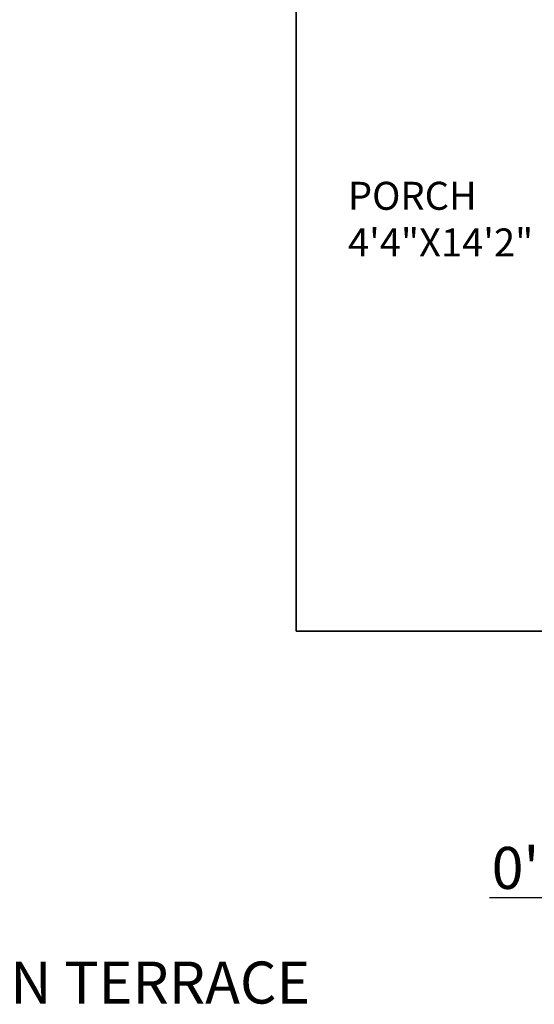
# Model space of a CAD drawing. Units: inches. Extents: x 3321 to 5237, y 11 to 1752.
# Tile 27 of 43: x 4881 to 4991, y 1345 to 1556. Entities that reach past the tile are written whole.
import ezdxf

# ---------------------------------------------------------------- set-up
doc = ezdxf.new("R2010")
doc.units = ezdxf.units.IN
for name, color, linetype, lineweight in [('A-ANNO-DIMS', 2, 'Continuous', 18), ('A-AREA-IDEN', 7, 'Continuous', 18), ('A-WALL', 7, 'Continuous', 35)]:
    doc.layers.add(name, color=color, linetype=linetype, lineweight=lineweight)
doc.styles.get("Standard").update_dxf_attribs({"font": 'arial.ttf'})
doc.dimstyles.new('ISO-25', dxfattribs={"dimtxt": 9, "dimasz": 2.5, "dimexe": 1.25, "dimexo": 0.625, "dimtad": 1, "dimdec": 1, "dimlunit": 3, "dimtxsty": 'Standard', "dimcen": 2.5, "dimclrd": 4, "dimclre": 4, "dimclrt": 256, "dimadec": 0, "dimazin": 0, "dimtfac": 1, "dimtdec": 1, "dimtmove": 0, "dimatfit": 3, "dimfxl": 1, "dimarcsym": 0})

# ---------------------------------------------------------------- blocks, each defined once
blk = doc.blocks.new('*D200')
at = {"layer": 'A-ANNO-DIMS', "color": 4, "lineweight": -2, "transparency": 16777216}
for p, q in [((5061.07, 1368.14), (4981.49, 1368.14)), ((5061.07, 1369.01), (5061.07, 1366.89)), ((5065.07, 1368.14), (5063.57, 1368.14)), ((5067.57, 1369.01), (5067.57, 1366.89))]:
    blk.add_line(p, q, dxfattribs=at)
at = {"layer": 'A-ANNO-DIMS', "color": 4, "transparency": 16777216}
for points in [[(5063.57, 1368.55), (5063.57, 1367.72), (5061.07, 1368.14)], [(5065.07, 1368.55), (5065.07, 1367.72), (5067.57, 1368.14)]]:
    blk.add_solid(points, dxfattribs=at)
at = {"layer": 'Defpoints', "color": 0, "transparency": 16777216}
for p in [(5061.07, 1369.64), (5067.57, 1369.64), (5061.07, 1368.14)]:
    blk.add_point(p, dxfattribs=at)
at = {"layer": 'A-ANNO-DIMS', "transparency": 16777216, "insert": (5020.03, 1373.41), "char_height": 9, "attachment_point": 5}
blk.add_mtext('0\'-6 1/2" TYP.', dxfattribs=at)

msp = doc.modelspace()

# ---------------------------------------------------------------- linework, layer by layer
at = {"layer": 'A-WALL'}
for p, q in [((4940.08, 1687.34), (4940.08, 1425.34)), ((4940.08, 1425.34), (5057.08, 1425.34))]:
    msp.add_line(p, q, dxfattribs=at)

# ---------------------------------------------------------------- texts
at = {"layer": 'A-AREA-IDEN', "attachment_point": 1}
for s, width, insert, char_height in [('PORCH\\P4\'4"X14\'2"', 97.3114, (4951.15, 1521.6), 6), ('OPEN TERRACE', 123.9378, (4854.62, 1354.51), 9)]:
    msp.add_mtext_dynamic_manual_height_columns(s, width=width, gutter_width=25, heights=[0], dxfattribs=dict(at, insert=insert, char_height=char_height))

# ---------------------------------------------------------------- dimensions: what is measured, and where the dimension line sits
at = {"layer": 'A-ANNO-DIMS'}
dim = msp.add_linear_dim(base=(5061.07, 1368.14), p1=(5067.57, 1369.64), p2=(5061.07, 1369.64), angle=180, text='<> TYP.', dimstyle='ISO-25', override={"dimdec": 1, "dimlfac": 1, "dimrnd": 0, "dimzin": 1, "dimdsep": 46, "dimlunit": 4, "dimfrac": 2}, dxfattribs=at)
dim.commit()
dim.dimension.update_dxf_attribs({"geometry": '*D200', "text_midpoint": (5020.03, 1373.41)})

doc.saveas('drawing.dxf')
